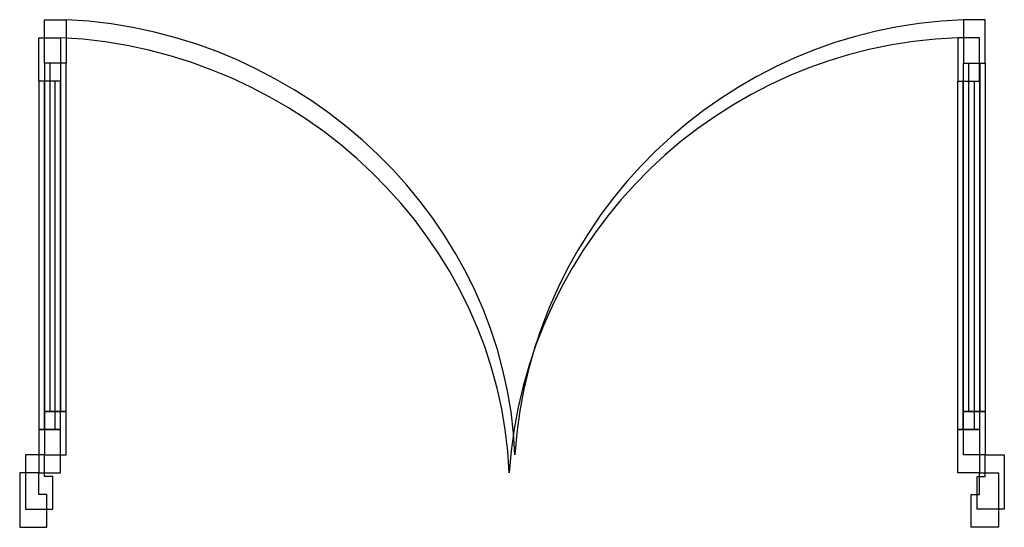
# Model space of a CAD drawing. Units: inches. Extents: x -43 to 8979, y -615 to 8149.
# Tile 4 of 5: x 7168 to 8979, y -488 to 445. Entities that reach past the tile are written whole.
import ezdxf

# ---------------------------------------------------------------- set-up
doc = ezdxf.new("R2010")
doc.units = ezdxf.units.IN
doc.layers.add('A-DOOR', color=4, linetype='Continuous', lineweight=25)

# ---------------------------------------------------------------- blocks, each defined once
blk = doc.blocks.new('A$C3628088D')
for p, q in [((35, 820), (35, 900)), ((35, 900), (75, 900)), ((75, 900), (75, 820)), ((75, 820), (35, 820)), ((75, 820), (35, 820)), ((35, 820), (35, 180)), ((45, 820), (45, 180)), ((65, 820), (45, 820)), ((65, 180), (65, 820)), ((75, 180), (75, 820)), ((35, 180), (35, 100)), ((75, 180), (35, 180)), ((35, 180), (75, 180)), ((45, 180), (65, 180)), ((75, 100), (75, 180)), ((35, 100), (0, 100)), ((0, 100), (0, 0)), ((35, 60), (35, 100)), ((35, 100), (75, 100)), ((50, 60), (35, 60)), ((50, 50), (50, 60)), ((50, 0), (50, 50)), ((0, 0), (50, 0))]:
    blk.add_line(p, q)
for points in [[(1725, 900), (1725, 820), (1765, 820), (1765, 900)], [(1725, 180), (1725, 820), (1765, 820), (1765, 180)], [(1735, 180), (1735, 820), (1755, 820), (1755, 180)], [(1725, 100), (1725, 180), (1765, 180), (1765, 100)], [(1765, 100), (1800, 100), (1800, 0), (1750, 0), (1750, 50), (1750, 60), (1765, 60)]]:
    blk.add_lwpolyline(points, close=True)
blk.add_arc((1756.5, 42.1), 858.5, 92.1038, 176.1334)
blk.add_ellipse((70, 105), major_axis=(-772.1, 325.5), ratio=0.94084, start_param=-2.726592, end_param=-1.199193)

msp = doc.modelspace()

# ---------------------------------------------------------------- block references
at = {"layer": 'A-DOOR'}
for p in [(7178.587, -455.111), (7167.937, -488.25)]:
    msp.add_blockref('A$C3628088D', p, dxfattribs=at)

doc.saveas('drawing.dxf')
